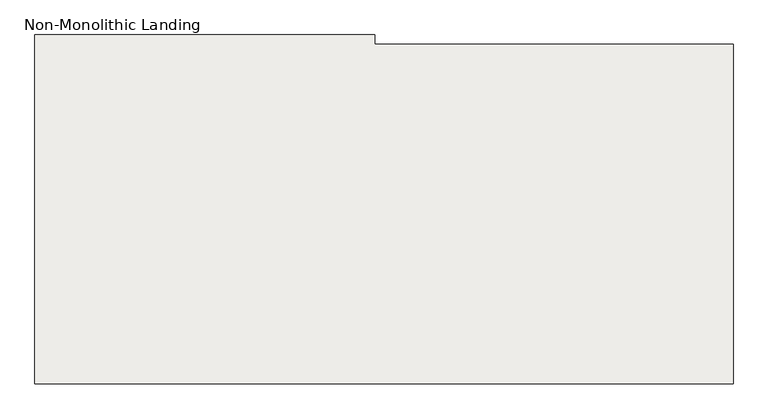
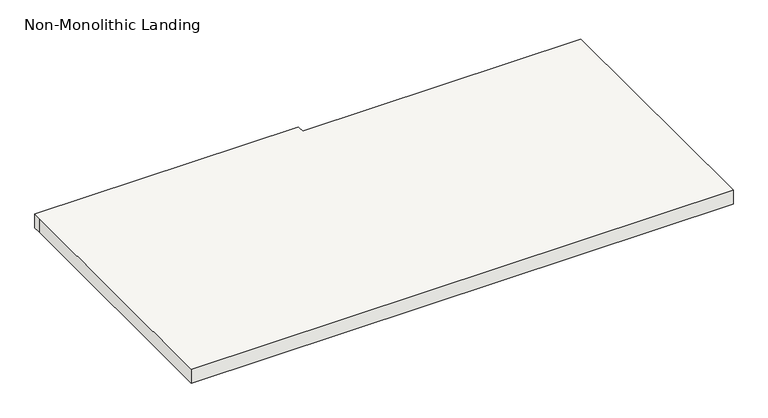
"""IFC4 building model written with IfcOpenShell, lengths in millimetres: slab geometry, Non-Monolithic Landing."""

from ifc_helpers import new_model, si_unit, origin, place, context, project, spatial, faceted_brep, source, transform, mapped, element, save


def non_monolithic_landing_daa301cf(model_context):
    return source(origin(), model_context, "Body", "Brep", [
        faceted_brep([(-3400.7137331, -6527.0593836, 11003.8118174), (-3400.7137331, -6552.4593836, 10978.4118174), (-4315.1137331, -6552.4593836, 10978.4118174), (-4315.1137331, -6527.0593836, 11003.8118174), (-4365.9137331, -6527.0593836, 11022.8618174), (-4365.9137331, -6501.6593836, 11022.8618174), (-5280.3137331, -6501.6593836, 11022.8618174), (-5280.3137331, -6527.0593836, 11022.8618174), (-5280.3137331, -7441.4593836, 11022.8618174), (-3400.7137331, -7441.4593836, 11022.8618174), (-3400.7137331, -6527.0593836, 11022.8618174), (-4315.1137331, -6552.4593836, 10972.0618174), (-3400.7137331, -6552.4593836, 10972.0618174), (-3400.7137331, -7441.4593836, 10972.0618174), (-5280.3137331, -7441.4593836, 10972.0618174), (-5280.3137331, -6527.0593836, 10972.0618174), (-5280.3137331, -6501.6593836, 10972.0618174), (-4365.9137331, -6501.6593836, 10972.0618174), (-4365.9137331, -6527.0593836, 10972.0618174), (-4315.1137331, -6527.0593836, 10972.0618174)], [[[0, 1, 2, 3]], [[4, 5, 6, 7, 8, 9, 10]], [[11, 12, 13, 14, 15, 16, 17, 18, 19]], [[12, 11, 2, 1]], [[11, 19, 3, 2]], [[4, 10, 0, 3, 19, 18]], [[5, 4, 18, 17]], [[6, 5, 17, 16]], [[7, 6, 16, 15]], [[8, 7, 15, 14]], [[9, 8, 14, 13]], [[10, 9, 13, 12, 1, 0]]]),
    ])


if __name__ == "__main__":
    model = new_model("IFC4")
    model_context = context("Model", 3, world=origin())
    ifc_project = project(units=[si_unit("LENGTHUNIT", "METRE", prefix="MILLI")], contexts=[model_context])
    site = spatial("IfcSite", under=ifc_project)
    building = spatial("IfcBuilding", under=site)
    placement = place(None, origin())
    non_monolithic_landing_shape = non_monolithic_landing_daa301cf(model_context)
    element("IfcSlab", 1, ObjectType="Non-Monolithic Landing", at=placement, inside=building, context=model_context, shape_type="MappedRepresentation", body=[
        mapped(non_monolithic_landing_shape, transform((0.0, 0.0, 0.0), x_axis=(1.0, 0.0, 0.0), y_axis=(0.0, 1.0, 0.0), z_axis=(0.0, 0.0, 1.0))),
    ])
    save(model, "model.ifc")
